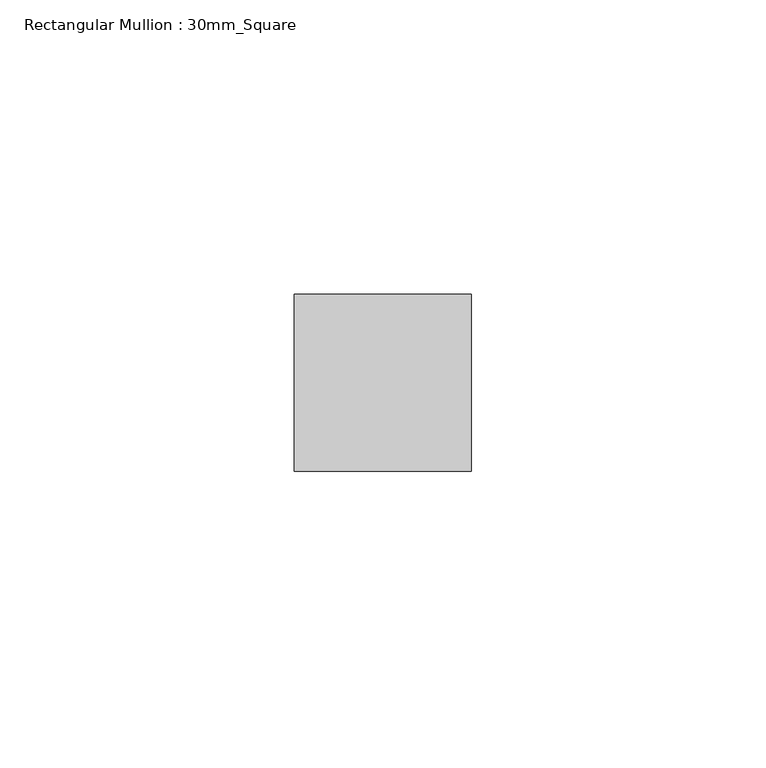
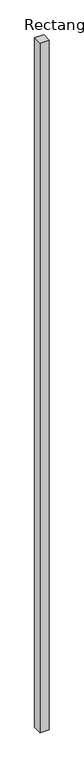
"""IFC4 building model written with IfcOpenShell, lengths in millimetres: member geometry, Rectangular Mullion : 30mm_Square."""

from ifc_helpers import new_model, si_unit, frame, origin, place, context, project, spatial, polyline, outline, extrude, source, transform, mapped, element, save


def rectangular_mullion_30mm_square_ff288ed3(model_context):
    return source(origin(), model_context, "Body", "SweptSolid", [
        extrude(outline(polyline([(15.0, 15.0), (15.0, -15.0), (-15.0, -15.0), (-15.0, 15.0), (15.0, 15.0)])), frame((0.0, 0.0, -2400.0242188), z_axis=(0.0, 0.0, 1.0), x_axis=(1.0, 0.0, 0.0)), (0.0, 0.0, 1.0), 2400.0242188),
    ])


if __name__ == "__main__":
    model = new_model("IFC4")
    model_context = context("Model", 3, world=origin())
    ifc_project = project(units=[si_unit("LENGTHUNIT", "METRE", prefix="MILLI")], contexts=[model_context])
    site = spatial("IfcSite", under=ifc_project)
    building = spatial("IfcBuilding", under=site)
    placement = place(None, origin())
    rectangular_mullion_30mm_square_shape = rectangular_mullion_30mm_square_ff288ed3(model_context)
    element("IfcMember", 1, ObjectType="Rectangular Mullion : 30mm_Square", at=placement, inside=building, context=model_context, shape_type="MappedRepresentation", body=[
        mapped(rectangular_mullion_30mm_square_shape, transform((0.0, 0.0, 0.0), x_axis=(1.0, 0.0, 0.0), y_axis=(0.0, 1.0, 0.0), z_axis=(0.0, 0.0, 1.0))),
    ])
    save(model, "model.ifc")

# Revit data of these elements
# Type "Rectangular Mullion : 30mm_Square"
#   Keynote = "H11"
#   built-in parameter 1007304 = 0.0984252 (stored number, unit not read)
#   built-in parameter 1007301 = 0.0492126 (stored number, unit not read)
#   built-in parameter 1007300 = 0.0492126 (stored number, unit not read)
# Element 1 (IfcMember, "Rectangular Mullion : 30mm_Square")
#   Materials on its faces: "Aluminium"
# Materials
#   "Aluminium": class "Metal", colour RGB 247 247 247, transparency 0, Description = "Aluminium 6061", Cost = 0
